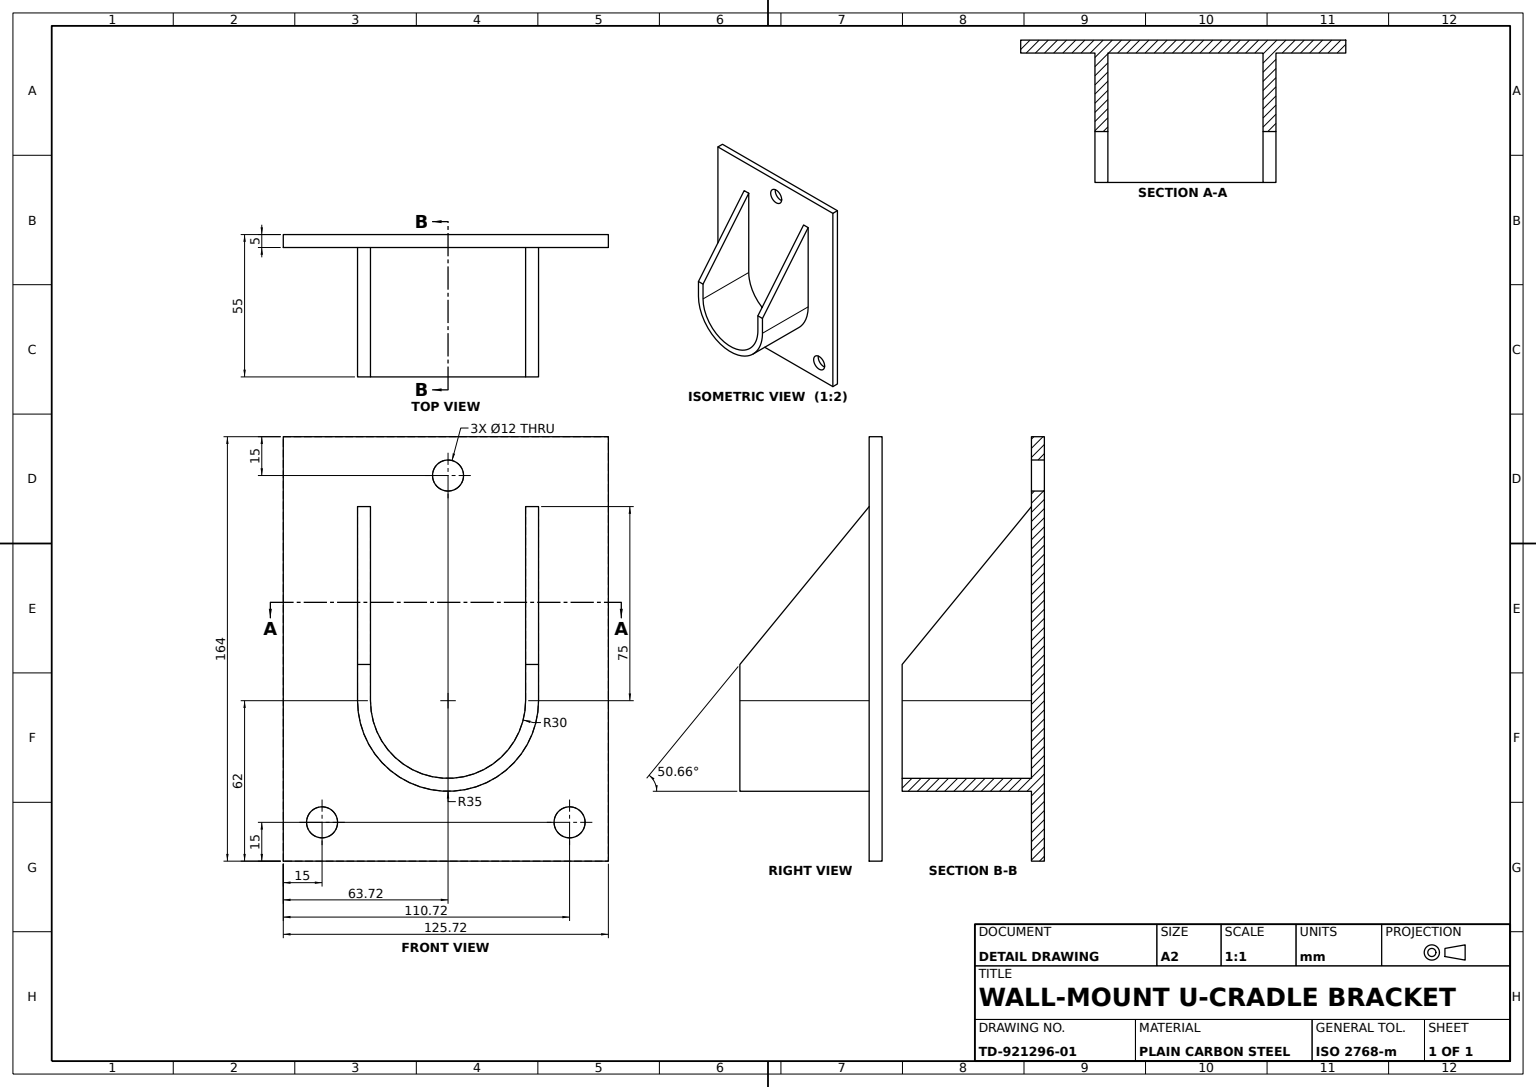
from build123d import *

# Parameters (mm, degrees)
U_CHANNEL_DEPTH         = 55
FLANGE_PLATE_SKETCH_W   = 125.717283216
FLANGE_PLATE_SKETCH_H   = 164
FLANGE_PLATE_SKETCH_R   = 6
FLANGE_PLATE_DEPTH      = 5
CHANNEL_SIDE_TRIM_DEPTH = 171.979049299


with BuildPart() as part:
    # U-Channel Profile Sketch → U-Channel (new body)
    with BuildSketch(Plane.XY):
        with BuildLine():
            Line((35, 0), (35, 75))
            Line((35, 75), (30, 75))
            Line((30, 75), (30, 0))
            ThreePointArc((30, 0), (0, -30), (-30, 0))
            Line((-30, 0), (-30, 75))
            Line((-30, 75), (-35, 75))
            Line((-35, 75), (-35, 0))
            ThreePointArc((-35, 0), (0, -35), (35, 0))
        make_face()
    extrude(amount=U_CHANNEL_DEPTH)

    # Flange Plate Sketch → Flange Plate (add)
    with BuildSketch(Plane(origin=(0, 0, 0), x_dir=(-1, 0, 0), z_dir=(0, 0, -1))):
        with Locations((0.858641608, 20)):
            Rectangle(FLANGE_PLATE_SKETCH_W, FLANGE_PLATE_SKETCH_H)
        with Locations((48.717283216, -47)):
            Circle(FLANGE_PLATE_SKETCH_R, mode=Mode.SUBTRACT)
        with Locations((-47, -47)):
            Circle(FLANGE_PLATE_SKETCH_R, mode=Mode.SUBTRACT)
        with Locations((0, 87)):
            Circle(FLANGE_PLATE_SKETCH_R, mode=Mode.SUBTRACT)
    extrude(amount=-FLANGE_PLATE_DEPTH)

    # Channel Side Trim Sketch → Channel Side Trim (cut, through all)
    with BuildSketch(Plane(origin=(62, 0, 0), x_dir=(0, 0, -1), z_dir=(1, 0, 0))):
        Polygon((-55, 14), (-5, 75), (-55, 75), align=None)
    extrude(amount=-CHANNEL_SIDE_TRIM_DEPTH, mode=Mode.SUBTRACT)


solid = part.part
